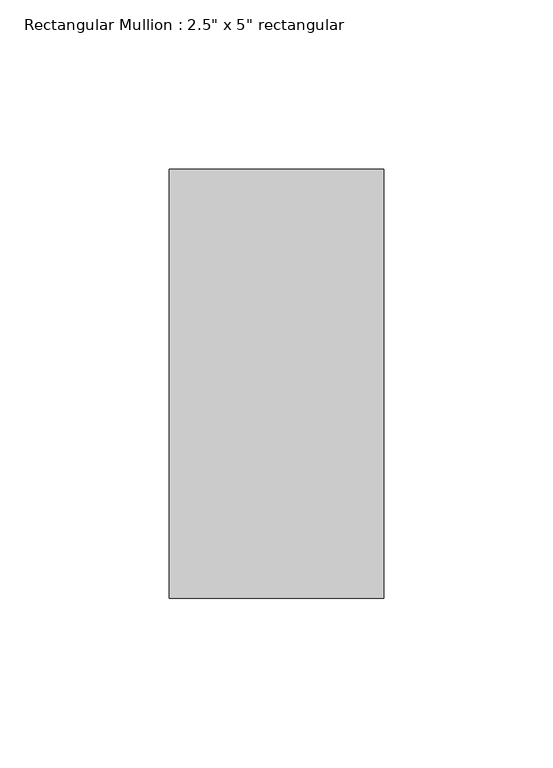
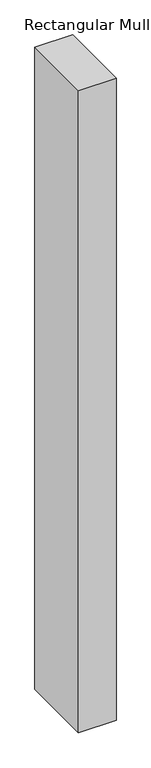
"""IFC4 building model written with IfcOpenShell, lengths in millimetres: member geometry."""

from ifc_helpers import new_model, si_unit, frame, origin, place, context, project, spatial, polyline, outline, extrude, source, transform, mapped, element, save


def member_a8f28920(model_context):
    return source(origin(), model_context, "Body", "SweptSolid", [
        extrude(outline(polyline([(0.0, 63.5), (0.0, -63.5), (-63.5, -63.5), (-63.5, 63.5), (0.0, 63.5)])), frame((0.0, 0.0, -1145.7631063), z_axis=(0.0, 0.0, 1.0), x_axis=(1.0, 0.0, 0.0)), (0.0, 0.0, 1.0), 1145.7631063),
    ])


if __name__ == "__main__":
    model = new_model("IFC4")
    model_context = context("Model", 3, world=origin())
    ifc_project = project(units=[si_unit("LENGTHUNIT", "METRE", prefix="MILLI")], contexts=[model_context])
    site = spatial("IfcSite", under=ifc_project)
    building = spatial("IfcBuilding", under=site)
    placement = place(None, origin())
    member_shape = member_a8f28920(model_context)
    element("IfcMember", 1, ObjectType="Rectangular Mullion : 2.5\" x 5\" rectangular", at=placement, inside=building, context=model_context, shape_type="MappedRepresentation", body=[
        mapped(member_shape, transform((0.0, 0.0, 0.0), x_axis=(1.0, 0.0, 0.0), y_axis=(0.0, 1.0, 0.0), z_axis=(0.0, 0.0, 1.0))),
    ])
    save(model, "model.ifc")

# Revit data of these elements
# Type "Rectangular Mullion : 2.5\" x 5\" rectangular"
#   built-in parameter 1007304 = 0.416667 (stored number, unit not read)
#   built-in parameter 1007301 = 0.104167 (stored number, unit not read)
#   built-in parameter 1007300 = 0.104167 (stored number, unit not read)
# Element 1 (IfcMember, "Rectangular Mullion : 2.5\" x 5\" rectangular")
#   Materials on its faces: "Aluminum"
# Materials
#   "Aluminum": class "Metal", colour RGB 247 247 247, transparency 0, Description = "Aluminum 6061", Cost = 0
